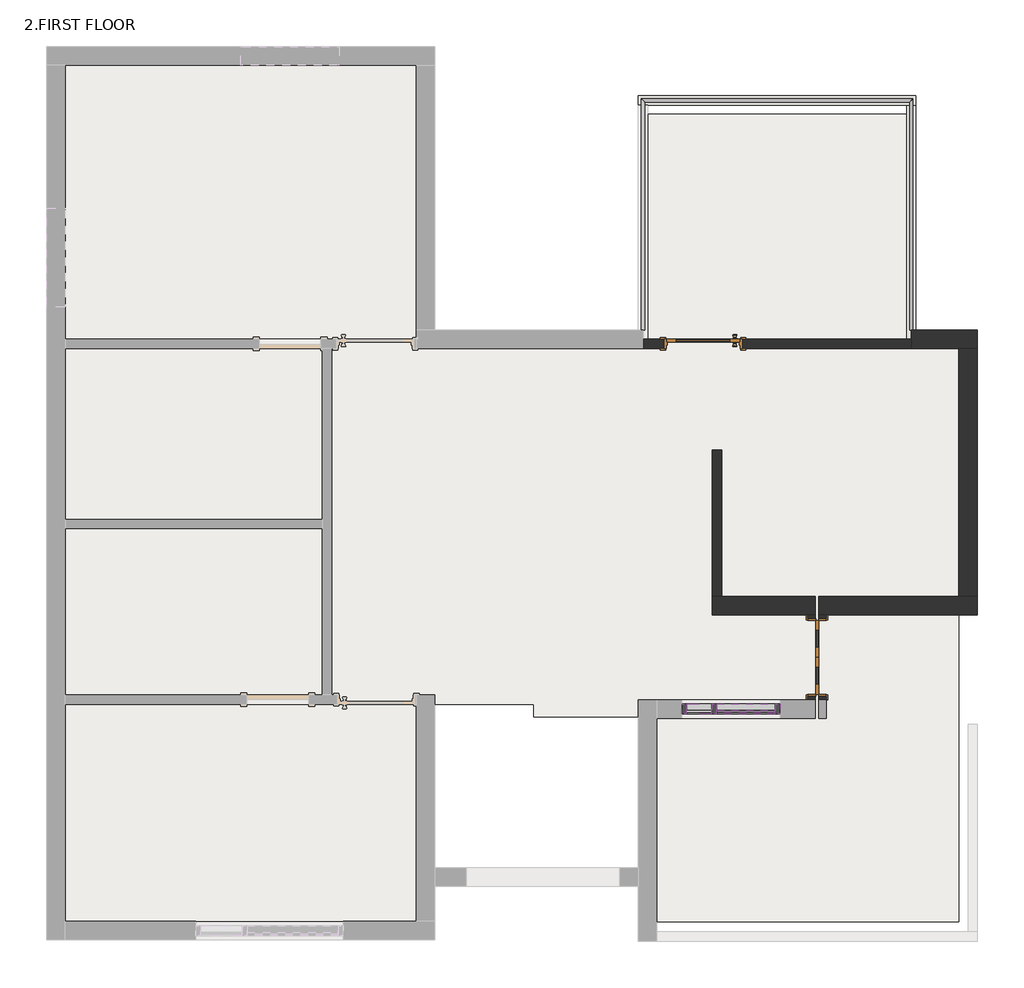
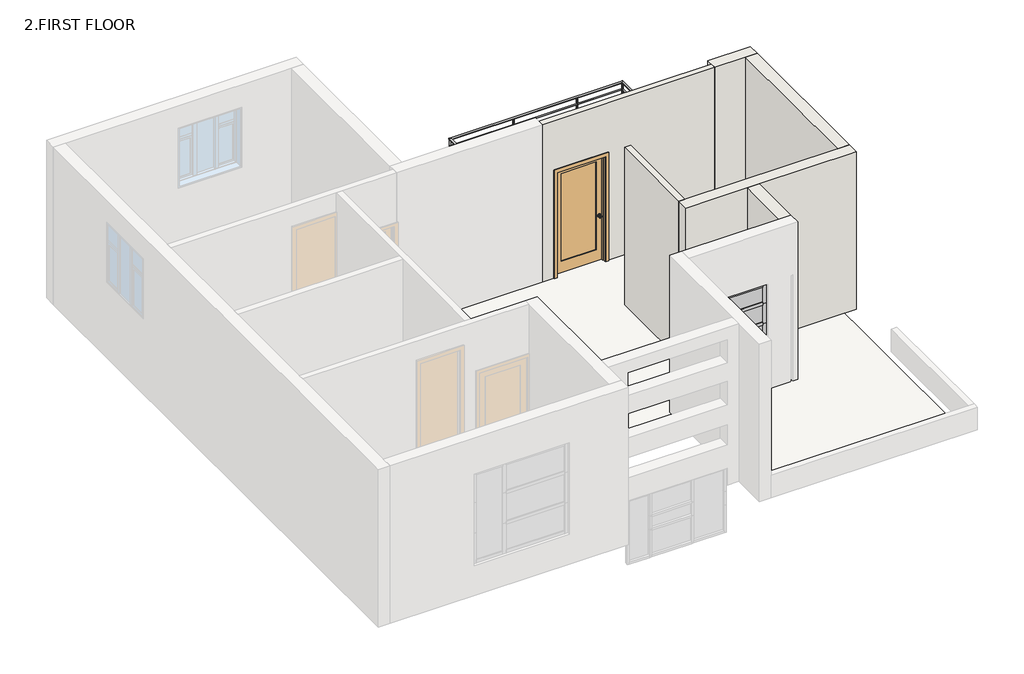
# One storey, part 2 of 2: 15 members, 8 walls, 3 plates, 2 doors, 1 railing, 1 slab.
"""IFC4 building model written with IfcOpenShell, lengths in millimetres."""

from ifc_helpers import new_model, si_unit, point, frame, frame_2d, origin, place, context, project, spatial, polyline, circle_curve, ellipse_curve, trimmed, segment, composite_curve, outline, extrude, faceted_brep, transform, mapped, element, save
from ifc_brep_helpers import plane_surface, cylinder_surface, advanced_brep
from components import door_interior_double_pocket_2_panel_wood_3_x_7_65f9ecc5, door_interior_single_1_panel_wood_4_x7_a3feeac7, member_5ad95953, member_7007ad49, member_90c805a2, member_abeaf8ac, member_7cfea1b5, system_panel_glazed_fef3bb39, system_panel_glazed_ef4f0122

model = new_model("IFC4")

# Units and contexts
model_context = context("Model", 3, world=origin())
ifc_project = project(units=[si_unit("LENGTHUNIT", "METRE", prefix="MILLI")], contexts=[model_context])

# Site, building, storey
site = spatial("IfcSite", under=ifc_project)
building = spatial("IfcBuilding", under=site)
storey = spatial("IfcBuildingStorey", under=building, Name="2.FIRST FLOOR", Elevation=3810.0)

# Doors
placement = place(None, origin())
door_interior_double_pocket_2_panel_wood_3_x_7_shape = door_interior_double_pocket_2_panel_wood_3_x_7_65f9ecc5(model_context)
element("IfcDoor", 1, ObjectType="Door-Interior-Double-Pocket-2_Panel-Wood : 3' x 7'", at=placement, inside=storey, context=model_context, shape_type="MappedRepresentation", body=[
    mapped(door_interior_double_pocket_2_panel_wood_3_x_7_shape, transform((1959.9250448, 2774.2910289, 3810.0), x_axis=(0.0, -1.0, 0.0), y_axis=(1.0, 0.0, 0.0), z_axis=(0.0, 0.0, 1.0))),
])
door_interior_single_1_panel_wood_4_x7_shape = door_interior_single_1_panel_wood_4_x7_a3feeac7(model_context)
element("IfcDoor", 2, ObjectType="Door-Interior-Single-1_Panel-Wood : 4'X7'", at=placement, inside=storey, context=model_context, shape_type="MappedRepresentation", body=[
    mapped(door_interior_single_1_panel_wood_4_x7_shape, transform((550.2250448, 6654.1410289, 3810.0), x_axis=(-1.0, 0.0, 0.0), y_axis=(0.0, -1.0, 0.0), z_axis=(0.0, 0.0, 1.0))),
])

# Members
member_shape = member_5ad95953(model_context)
element("IfcMember", 3, ObjectType="Rectangular Mullion : 2.5\" x 5\" rectangular", at=placement, inside=storey, context=model_context, shape_type="MappedRepresentation", body=[
    mapped(member_shape, transform((347.0250448, 2136.1160289, 5943.6), x_axis=(0.0, 0.0, 1.0), y_axis=(0.0, 1.0, 0.0), z_axis=(-1.0, 0.0, 0.0))),
])
member_2_shape = member_7007ad49(model_context)
element("IfcMember", 4, ObjectType="Rectangular Mullion : 2.5\" x 5\" rectangular", at=placement, inside=storey, context=model_context, shape_type="MappedRepresentation", body=[
    mapped(member_2_shape, transform((1439.2250448, 2136.1160289, 4724.4), x_axis=(0.0, 0.0, -1.0), y_axis=(0.0, 1.0, 0.0), z_axis=(1.0, 0.0, 0.0))),
])
member_3_shape = member_90c805a2(model_context)
element("IfcMember", 5, ObjectType="Rectangular Mullion : 2.5\" x 5\" rectangular", at=placement, inside=storey, context=model_context, shape_type="MappedRepresentation", body=[
    mapped(member_3_shape, transform((689.9250448, 2136.1160289, 4724.4), x_axis=(-1.0, 0.0, 0.0), y_axis=(0.0, 1.0, 0.0), z_axis=(0.0, 0.0, -1.0))),
])
member_4_shape = member_abeaf8ac(model_context)
element("IfcMember", 6, ObjectType="Rectangular Mullion : 2.5\" x 5\" rectangular", at=placement, inside=storey, context=model_context, shape_type="MappedRepresentation", body=[
    mapped(member_4_shape, transform((721.6750448, 2136.1160289, 5537.2), x_axis=(0.0, 0.0, 1.0), y_axis=(0.0, 1.0, 0.0), z_axis=(-1.0, 0.0, 0.0))),
])
element("IfcMember", 7, ObjectType="Rectangular Mullion : 2.5\" x 5\" rectangular", at=placement, inside=storey, context=model_context, shape_type="MappedRepresentation", body=[
    mapped(member_4_shape, transform((721.6750448, 2136.1160289, 5130.8), x_axis=(0.0, 0.0, 1.0), y_axis=(0.0, 1.0, 0.0), z_axis=(-1.0, 0.0, 0.0))),
])
element("IfcMember", 8, ObjectType="Rectangular Mullion : 2.5\" x 5\" rectangular", at=placement, inside=storey, context=model_context, shape_type="MappedRepresentation", body=[
    mapped(member_shape, transform((658.1750448, 2136.1160289, 4724.4), x_axis=(0.0, 0.0, -1.0), y_axis=(0.0, 1.0, 0.0), z_axis=(1.0, 0.0, 0.0))),
])
element("IfcMember", 9, ObjectType="Rectangular Mullion : 2.5\" x 5\" rectangular", at=placement, inside=storey, context=model_context, shape_type="MappedRepresentation", body=[
    mapped(member_2_shape, transform((721.6750448, 2136.1160289, 5943.6), x_axis=(0.0, 0.0, 1.0), y_axis=(0.0, 1.0, 0.0), z_axis=(-1.0, 0.0, 0.0))),
])
element("IfcMember", 10, ObjectType="Rectangular Mullion : 2.5\" x 5\" rectangular", at=placement, inside=storey, context=model_context, shape_type="MappedRepresentation", body=[
    mapped(member_3_shape, transform((689.9250448, 2136.1160289, 5537.2), x_axis=(-1.0, 0.0, 0.0), y_axis=(0.0, 1.0, 0.0), z_axis=(0.0, 0.0, -1.0))),
])
element("IfcMember", 11, ObjectType="Rectangular Mullion : 2.5\" x 5\" rectangular", at=placement, inside=storey, context=model_context, shape_type="MappedRepresentation", body=[
    mapped(member_3_shape, transform((689.9250448, 2136.1160289, 5130.8), x_axis=(-1.0, 0.0, 0.0), y_axis=(0.0, 1.0, 0.0), z_axis=(0.0, 0.0, -1.0))),
])
member_5_shape = member_7cfea1b5(model_context)
element("IfcMember", 12, ObjectType="Rectangular Mullion : 2.5\" x 5\" rectangular", at=placement, inside=storey, context=model_context, shape_type="MappedRepresentation", body=[
    mapped(member_5_shape, transform((1502.7250448, 2136.1160289, 5943.6), x_axis=(1.0, 0.0, 0.0), y_axis=(0.0, 1.0, 0.0), z_axis=(0.0, 0.0, 1.0))),
])
element("IfcMember", 13, ObjectType="Rectangular Mullion : 2.5\" x 5\" rectangular", at=placement, inside=storey, context=model_context, shape_type="MappedRepresentation", body=[
    mapped(member_5_shape, transform((283.5250448, 2136.1160289, 4724.4), x_axis=(-1.0, 0.0, 0.0), y_axis=(0.0, 1.0, 0.0), z_axis=(0.0, 0.0, -1.0))),
])
element("IfcMember", 14, ObjectType="Rectangular Mullion : 2.5\" x 5\" rectangular", at=placement, inside=storey, context=model_context, shape_type="MappedRepresentation", body=[
    mapped(member_5_shape, transform((283.5250448, 2136.1160289, 5537.2), x_axis=(-1.0, 0.0, 0.0), y_axis=(0.0, 1.0, 0.0), z_axis=(0.0, 0.0, -1.0))),
])
element("IfcMember", 15, ObjectType="Rectangular Mullion : 2.5\" x 5\" rectangular", at=placement, inside=storey, context=model_context, shape_type="MappedRepresentation", body=[
    mapped(member_5_shape, transform((283.5250448, 2136.1160289, 5130.8), x_axis=(-1.0, 0.0, 0.0), y_axis=(0.0, 1.0, 0.0), z_axis=(0.0, 0.0, -1.0))),
])
element("IfcMember", 16, ObjectType="Rectangular Mullion : 2.5\" x 5\" rectangular", at=placement, inside=storey, context=model_context, shape_type="MappedRepresentation", body=[
    mapped(member_5_shape, transform((1502.7250448, 2136.1160289, 5537.2), x_axis=(1.0, 0.0, 0.0), y_axis=(0.0, 1.0, 0.0), z_axis=(0.0, 0.0, 1.0))),
])
element("IfcMember", 17, ObjectType="Rectangular Mullion : 2.5\" x 5\" rectangular", at=placement, inside=storey, context=model_context, shape_type="MappedRepresentation", body=[
    mapped(member_5_shape, transform((1502.7250448, 2136.1160289, 5130.8), x_axis=(1.0, 0.0, 0.0), y_axis=(0.0, 1.0, 0.0), z_axis=(0.0, 0.0, 1.0))),
])

# Plates
system_panel_glazed_shape = system_panel_glazed_fef3bb39(model_context)
element("IfcPlate", 18, ObjectType="System Panel : Glazed", at=placement, inside=storey, context=model_context, shape_type="MappedRepresentation", body=[
    mapped(system_panel_glazed_shape, transform((1080.4500448, 2136.1160289, 4787.9), x_axis=(-1.0, 0.0, 0.0), y_axis=(0.0, -1.0, 0.0), z_axis=(0.0, 0.0, 1.0))),
])
element("IfcPlate", 19, ObjectType="System Panel : Glazed", at=placement, inside=storey, context=model_context, shape_type="MappedRepresentation", body=[
    mapped(system_panel_glazed_shape, transform((1080.4500448, 2136.1160289, 5568.95), x_axis=(-1.0, 0.0, 0.0), y_axis=(0.0, -1.0, 0.0), z_axis=(0.0, 0.0, 1.0))),
])
system_panel_glazed_2_shape = system_panel_glazed_ef4f0122(model_context)
element("IfcPlate", 20, ObjectType="System Panel : Glazed", at=placement, inside=storey, context=model_context, shape_type="MappedRepresentation", body=[
    mapped(system_panel_glazed_2_shape, transform((1080.4500448, 2136.1160289, 5162.55), x_axis=(-1.0, 0.0, 0.0), y_axis=(0.0, -1.0, 0.0), z_axis=(0.0, 0.0, 1.0))),
])

# Railing
element("IfcRailing", 21, ObjectType="Handrail - Pipe", at=placement, inside=storey, context=model_context, shape_type="SolidModel", body=[
    advanced_brep(
    [(-173.6749552, 6822.4160289, 4857.75), (-211.7749552, 6822.4160289, 4857.75), (3102.9250448, 6822.4160289, 4857.75), (3141.0250448, 6822.4160289, 4857.75), (-173.6749552, 9641.8160289, 4857.75), (-211.7749552, 9679.9160289, 4857.75), (3102.9250448, 9641.8160289, 4857.75), (3141.0250448, 9679.9160289, 4857.75)],
    [
        (0, 1, circle_curve(frame((-192.7249552, 6822.4160289, 4857.75), z_axis=(0.0, -1.0, 0.0), x_axis=(-1.0, 0.0, 0.0)), 19.05)),
        (1, 0, circle_curve(frame((-192.7249552, 6822.4160289, 4857.75), z_axis=(0.0, -1.0, 0.0), x_axis=(-1.0, 0.0, 0.0)), 19.05)),
        (2, 3, circle_curve(frame((3121.9750448, 6822.4160289, 4857.75), z_axis=(0.0, -1.0, 0.0), x_axis=(1.0, 0.0, 0.0)), 19.05)),
        (3, 2, circle_curve(frame((3121.9750448, 6822.4160289, 4857.75), z_axis=(0.0, -1.0, 0.0), x_axis=(1.0, 0.0, 0.0)), 19.05)),
        (0, 4),
        (4, 5, ellipse_curve(frame((-192.7249552, 9660.8660289, 4857.75), z_axis=(-0.7071067811865492, -0.7071067811865458, 0.0), x_axis=(0.7071067811865457, -0.7071067811865492, 0.0)), 26.9407684, 19.05)),
        (5, 1),
        (5, 4, ellipse_curve(frame((-192.7249552, 9660.8660289, 4857.75), z_axis=(-0.7071067811865492, -0.7071067811865458, 0.0), x_axis=(0.7071067811865457, -0.7071067811865492, 0.0)), 26.9407684, 19.05)),
        (4, 6),
        (6, 7, ellipse_curve(frame((3121.9750448, 9660.8660289, 4857.75), z_axis=(-0.7071067811865457, 0.7071067811865492, 0.0), x_axis=(-0.7071067811865493, -0.7071067811865457, 0.0)), 26.9407684, 19.05)),
        (7, 5),
        (7, 6, ellipse_curve(frame((3121.9750448, 9660.8660289, 4857.75), z_axis=(-0.7071067811865457, 0.7071067811865492, 0.0), x_axis=(-0.7071067811865493, -0.7071067811865457, 0.0)), 26.9407684, 19.05)),
        (6, 2),
        (3, 7),
    ],
    [
        plane_surface(frame((-192.7249552, 6822.4160289, 4876.8), z_axis=(0.0, -1.0, 0.0), x_axis=(0.0, 0.0, 1.0))),
        plane_surface(frame((3121.9750448, 6822.4160289, 4876.8), z_axis=(0.0, -1.0, 0.0), x_axis=(0.0, 0.0, -1.0))),
        cylinder_surface(frame((-192.7249552, 6822.4160289, 4857.75), z_axis=(0.0, -1.0, 0.0), x_axis=(-1.0, 0.0, 0.0)), 19.05),
        cylinder_surface(frame((-192.7249552, 9660.8660289, 4857.75), z_axis=(-1.0, 0.0, 0.0), x_axis=(0.0, 1.0, 0.0)), 19.05),
        cylinder_surface(frame((3121.9750448, 9660.8660289, 4857.75), z_axis=(0.0, 1.0, 0.0), x_axis=(1.0, 0.0, 0.0)), 19.05),
    ],
    [
        (0, [[1, 2]]),
        (1, [[3, 4]]),
        (2, [[-1, 5, 6, 7]]),
        (2, [[-2, -7, 8, -5]]),
        (3, [[-6, 9, 10, 11]]),
        (3, [[-8, -11, 12, -9]]),
        (4, [[-10, 13, -4, 14]]),
        (4, [[-12, -14, -3, -13]]),
    ],
),
    advanced_brep(
    [(-205.4249552, 6822.4160289, 4711.7), (-180.0249552, 6822.4160289, 4711.7), (3134.6750448, 6822.4160289, 4711.7), (3109.2750448, 6822.4160289, 4711.7), (-205.4249552, 9673.5660289, 4711.7), (-180.0249552, 9648.1660289, 4711.7), (3134.6750448, 9673.5660289, 4711.7), (3109.2750448, 9648.1660289, 4711.7)],
    [
        (0, 1, circle_curve(frame((-192.7249552, 6822.4160289, 4711.7), z_axis=(0.0, -1.0, 0.0), x_axis=(1.0, 0.0, 0.0)), 12.7)),
        (1, 0, circle_curve(frame((-192.7249552, 6822.4160289, 4711.7), z_axis=(0.0, -1.0, 0.0), x_axis=(1.0, 0.0, 0.0)), 12.7)),
        (2, 3, circle_curve(frame((3121.9750448, 6822.4160289, 4711.7), z_axis=(0.0, -1.0, 0.0), x_axis=(-1.0, 0.0, 0.0)), 12.7)),
        (3, 2, circle_curve(frame((3121.9750448, 6822.4160289, 4711.7), z_axis=(0.0, -1.0, 0.0), x_axis=(-1.0, 0.0, 0.0)), 12.7)),
        (0, 4),
        (4, 5, ellipse_curve(frame((-192.7249552, 9660.8660289, 4711.7), z_axis=(-0.7071067811865492, -0.7071067811865458, 0.0), x_axis=(0.7071067811865457, -0.7071067811865492, 0.0)), 17.9605122, 12.7)),
        (5, 1),
        (5, 4, ellipse_curve(frame((-192.7249552, 9660.8660289, 4711.7), z_axis=(-0.7071067811865492, -0.7071067811865458, 0.0), x_axis=(0.7071067811865457, -0.7071067811865492, 0.0)), 17.9605122, 12.7)),
        (4, 6),
        (6, 7, ellipse_curve(frame((3121.9750448, 9660.8660289, 4711.7), z_axis=(-0.7071067811865457, 0.7071067811865492, 0.0), x_axis=(-0.7071067811865493, -0.7071067811865457, 0.0)), 17.9605122, 12.7)),
        (7, 5),
        (7, 6, ellipse_curve(frame((3121.9750448, 9660.8660289, 4711.7), z_axis=(-0.7071067811865457, 0.7071067811865492, 0.0), x_axis=(-0.7071067811865493, -0.7071067811865457, 0.0)), 17.9605122, 12.7)),
        (6, 2),
        (3, 7),
    ],
    [
        plane_surface(frame((-192.7249552, 6822.4160289, 4724.4), z_axis=(0.0, -1.0, 0.0), x_axis=(0.0, 0.0, 1.0))),
        plane_surface(frame((3121.9750448, 6822.4160289, 4724.4), z_axis=(0.0, -1.0, 0.0), x_axis=(0.0, 0.0, -1.0))),
        cylinder_surface(frame((-192.7249552, 6822.4160289, 4711.7), z_axis=(0.0, -1.0, 0.0), x_axis=(1.0, 0.0, 0.0)), 12.7),
        cylinder_surface(frame((-192.7249552, 9660.8660289, 4711.7), z_axis=(-1.0, 0.0, 0.0), x_axis=(0.0, -1.0, 0.0)), 12.7),
        cylinder_surface(frame((3121.9750448, 9660.8660289, 4711.7), z_axis=(0.0, 1.0, 0.0), x_axis=(-1.0, 0.0, 0.0)), 12.7),
    ],
    [
        (0, [[1, 2]]),
        (1, [[3, 4]]),
        (2, [[-1, 5, 6, 7]]),
        (2, [[-2, -7, 8, -5]]),
        (3, [[-6, 9, 10, 11]]),
        (3, [[-8, -11, 12, -9]]),
        (4, [[-10, 13, -4, 14]]),
        (4, [[-12, -14, -3, -13]]),
    ],
),
    advanced_brep(
    [(-205.4249552, 6822.4160289, 4559.3), (-180.0249552, 6822.4160289, 4559.3), (3134.6750448, 6822.4160289, 4559.3), (3109.2750448, 6822.4160289, 4559.3), (-205.4249552, 9673.5660289, 4559.3), (-180.0249552, 9648.1660289, 4559.3), (3134.6750448, 9673.5660289, 4559.3), (3109.2750448, 9648.1660289, 4559.3)],
    [
        (0, 1, circle_curve(frame((-192.7249552, 6822.4160289, 4559.3), z_axis=(0.0, -1.0, 0.0), x_axis=(1.0, 0.0, 0.0)), 12.7)),
        (1, 0, circle_curve(frame((-192.7249552, 6822.4160289, 4559.3), z_axis=(0.0, -1.0, 0.0), x_axis=(1.0, 0.0, 0.0)), 12.7)),
        (2, 3, circle_curve(frame((3121.9750448, 6822.4160289, 4559.3), z_axis=(0.0, -1.0, 0.0), x_axis=(-1.0, 0.0, 0.0)), 12.7)),
        (3, 2, circle_curve(frame((3121.9750448, 6822.4160289, 4559.3), z_axis=(0.0, -1.0, 0.0), x_axis=(-1.0, 0.0, 0.0)), 12.7)),
        (0, 4),
        (4, 5, ellipse_curve(frame((-192.7249552, 9660.8660289, 4559.3), z_axis=(-0.7071067811865492, -0.7071067811865458, 0.0), x_axis=(0.7071067811865457, -0.7071067811865492, 0.0)), 17.9605122, 12.7)),
        (5, 1),
        (5, 4, ellipse_curve(frame((-192.7249552, 9660.8660289, 4559.3), z_axis=(-0.7071067811865492, -0.7071067811865458, 0.0), x_axis=(0.7071067811865457, -0.7071067811865492, 0.0)), 17.9605122, 12.7)),
        (4, 6),
        (6, 7, ellipse_curve(frame((3121.9750448, 9660.8660289, 4559.3), z_axis=(-0.7071067811865457, 0.7071067811865492, 0.0), x_axis=(-0.7071067811865493, -0.7071067811865457, 0.0)), 17.9605122, 12.7)),
        (7, 5),
        (7, 6, ellipse_curve(frame((3121.9750448, 9660.8660289, 4559.3), z_axis=(-0.7071067811865457, 0.7071067811865492, 0.0), x_axis=(-0.7071067811865493, -0.7071067811865457, 0.0)), 17.9605122, 12.7)),
        (6, 2),
        (3, 7),
    ],
    [
        plane_surface(frame((-192.7249552, 6822.4160289, 4572.0), z_axis=(0.0, -1.0, 0.0), x_axis=(0.0, 0.0, 1.0))),
        plane_surface(frame((3121.9750448, 6822.4160289, 4572.0), z_axis=(0.0, -1.0, 0.0), x_axis=(0.0, 0.0, -1.0))),
        cylinder_surface(frame((-192.7249552, 6822.4160289, 4559.3), z_axis=(0.0, -1.0, 0.0), x_axis=(1.0, 0.0, 0.0)), 12.7),
        cylinder_surface(frame((-192.7249552, 9660.8660289, 4559.3), z_axis=(-1.0, 0.0, 0.0), x_axis=(0.0, -1.0, 0.0)), 12.7),
        cylinder_surface(frame((3121.9750448, 9660.8660289, 4559.3), z_axis=(0.0, 1.0, 0.0), x_axis=(-1.0, 0.0, 0.0)), 12.7),
    ],
    [
        (0, [[1, 2]]),
        (1, [[3, 4]]),
        (2, [[-1, 5, 6, 7]]),
        (2, [[-2, -7, 8, -5]]),
        (3, [[-6, 9, 10, 11]]),
        (3, [[-8, -11, 12, -9]]),
        (4, [[-10, 13, -4, 14]]),
        (4, [[-12, -14, -3, -13]]),
    ],
),
    advanced_brep(
    [(-205.4249552, 6822.4160289, 4406.9), (-180.0249552, 6822.4160289, 4406.9), (-205.4249552, 9673.5660289, 4406.9), (-180.0249552, 9648.1660289, 4406.9), (3134.6750448, 9673.5660289, 4406.9), (3109.2750448, 9648.1660289, 4406.9), (3134.6750448, 6822.4160289, 4406.9), (3109.2750448, 6822.4160289, 4406.9)],
    [
        (0, 1, circle_curve(frame((-192.7249552, 6822.4160289, 4406.9), z_axis=(0.0, -1.0, 0.0), x_axis=(1.0, 0.0, 0.0)), 12.7)),
        (1, 0, circle_curve(frame((-192.7249552, 6822.4160289, 4406.9), z_axis=(0.0, -1.0, 0.0), x_axis=(1.0, 0.0, 0.0)), 12.7)),
        (0, 2),
        (2, 3, ellipse_curve(frame((-192.7249552, 9660.8660289, 4406.9), z_axis=(-0.7071067811865492, -0.7071067811865458, 0.0), x_axis=(0.7071067811865457, -0.7071067811865492, 0.0)), 17.9605122, 12.7)),
        (3, 1),
        (3, 2, ellipse_curve(frame((-192.7249552, 9660.8660289, 4406.9), z_axis=(-0.7071067811865492, -0.7071067811865458, 0.0), x_axis=(0.7071067811865457, -0.7071067811865492, 0.0)), 17.9605122, 12.7)),
        (2, 4),
        (4, 5, ellipse_curve(frame((3121.9750448, 9660.8660289, 4406.9), z_axis=(-0.7071067811865457, 0.7071067811865492, 0.0), x_axis=(-0.7071067811865493, -0.7071067811865457, 0.0)), 17.9605122, 12.7)),
        (5, 3),
        (5, 4, ellipse_curve(frame((3121.9750448, 9660.8660289, 4406.9), z_axis=(-0.7071067811865457, 0.7071067811865492, 0.0), x_axis=(-0.7071067811865493, -0.7071067811865457, 0.0)), 17.9605122, 12.7)),
        (6, 7, circle_curve(frame((3121.9750448, 6822.4160289, 4406.9), z_axis=(0.0, -1.0, 0.0), x_axis=(-1.0, 0.0, 0.0)), 12.7)),
        (7, 6, circle_curve(frame((3121.9750448, 6822.4160289, 4406.9), z_axis=(0.0, -1.0, 0.0), x_axis=(-1.0, 0.0, 0.0)), 12.7)),
        (4, 6),
        (7, 5),
    ],
    [
        plane_surface(frame((-192.7249552, 6822.4160289, 4419.6), z_axis=(0.0, -1.0, 0.0), x_axis=(0.0, 0.0, 1.0))),
        cylinder_surface(frame((-192.7249552, 6822.4160289, 4406.9), z_axis=(0.0, -1.0, 0.0), x_axis=(1.0, 0.0, 0.0)), 12.7),
        cylinder_surface(frame((-192.7249552, 9660.8660289, 4406.9), z_axis=(-1.0, 0.0, 0.0), x_axis=(0.0, -1.0, 0.0)), 12.7),
        plane_surface(frame((3121.9750448, 6822.4160289, 4419.6), z_axis=(0.0, -1.0, 0.0), x_axis=(0.0, 0.0, -1.0))),
        cylinder_surface(frame((3121.9750448, 9660.8660289, 4406.9), z_axis=(0.0, 1.0, 0.0), x_axis=(-1.0, 0.0, 0.0)), 12.7),
    ],
    [
        (0, [[1, 2]]),
        (1, [[-1, 3, 4, 5]]),
        (1, [[-2, -5, 6, -3]]),
        (2, [[-4, 7, 8, 9]]),
        (2, [[-6, -9, 10, -7]]),
        (3, [[11, 12]]),
        (4, [[-8, 13, -12, 14]]),
        (4, [[-10, -14, -11, -13]]),
    ],
),
    advanced_brep(
    [(-205.4249552, 6822.4160289, 4254.5), (-180.0249552, 6822.4160289, 4254.5), (-205.4249552, 9673.5660289, 4254.5), (-180.0249552, 9648.1660289, 4254.5), (3134.6750448, 9673.5660289, 4254.5), (3109.2750448, 9648.1660289, 4254.5), (3134.6750448, 6822.4160289, 4254.5), (3109.2750448, 6822.4160289, 4254.5)],
    [
        (0, 1, circle_curve(frame((-192.7249552, 6822.4160289, 4254.5), z_axis=(0.0, -1.0, 0.0), x_axis=(1.0, 0.0, 0.0)), 12.7)),
        (1, 0, circle_curve(frame((-192.7249552, 6822.4160289, 4254.5), z_axis=(0.0, -1.0, 0.0), x_axis=(1.0, 0.0, 0.0)), 12.7)),
        (0, 2),
        (2, 3, ellipse_curve(frame((-192.7249552, 9660.8660289, 4254.5), z_axis=(-0.7071067811865492, -0.7071067811865458, 0.0), x_axis=(0.7071067811865457, -0.7071067811865492, 0.0)), 17.9605122, 12.7)),
        (3, 1),
        (3, 2, ellipse_curve(frame((-192.7249552, 9660.8660289, 4254.5), z_axis=(-0.7071067811865492, -0.7071067811865458, 0.0), x_axis=(0.7071067811865457, -0.7071067811865492, 0.0)), 17.9605122, 12.7)),
        (2, 4),
        (4, 5, ellipse_curve(frame((3121.9750448, 9660.8660289, 4254.5), z_axis=(-0.7071067811865457, 0.7071067811865492, 0.0), x_axis=(-0.7071067811865493, -0.7071067811865457, 0.0)), 17.9605122, 12.7)),
        (5, 3),
        (5, 4, ellipse_curve(frame((3121.9750448, 9660.8660289, 4254.5), z_axis=(-0.7071067811865457, 0.7071067811865492, 0.0), x_axis=(-0.7071067811865493, -0.7071067811865457, 0.0)), 17.9605122, 12.7)),
        (6, 7, circle_curve(frame((3121.9750448, 6822.4160289, 4254.5), z_axis=(0.0, -1.0, 0.0), x_axis=(-1.0, 0.0, 0.0)), 12.7)),
        (7, 6, circle_curve(frame((3121.9750448, 6822.4160289, 4254.5), z_axis=(0.0, -1.0, 0.0), x_axis=(-1.0, 0.0, 0.0)), 12.7)),
        (4, 6),
        (7, 5),
    ],
    [
        plane_surface(frame((-192.7249552, 6822.4160289, 4267.2), z_axis=(0.0, -1.0, 0.0), x_axis=(0.0, 0.0, 1.0))),
        cylinder_surface(frame((-192.7249552, 6822.4160289, 4254.5), z_axis=(0.0, -1.0, 0.0), x_axis=(1.0, 0.0, 0.0)), 12.7),
        cylinder_surface(frame((-192.7249552, 9660.8660289, 4254.5), z_axis=(-1.0, 0.0, 0.0), x_axis=(0.0, -1.0, 0.0)), 12.7),
        plane_surface(frame((3121.9750448, 6822.4160289, 4267.2), z_axis=(0.0, -1.0, 0.0), x_axis=(0.0, 0.0, -1.0))),
        cylinder_surface(frame((3121.9750448, 9660.8660289, 4254.5), z_axis=(0.0, 1.0, 0.0), x_axis=(-1.0, 0.0, 0.0)), 12.7),
    ],
    [
        (0, [[1, 2]]),
        (1, [[-1, 3, 4, 5]]),
        (1, [[-2, -5, 6, -3]]),
        (2, [[-4, 7, 8, 9]]),
        (2, [[-6, -9, 10, -7]]),
        (3, [[11, 12]]),
        (4, [[-8, 13, -12, 14]]),
        (4, [[-10, -14, -11, -13]]),
    ],
),
    advanced_brep(
    [(-205.4249552, 6822.4160289, 4102.1), (-180.0249552, 6822.4160289, 4102.1), (-205.4249552, 9673.5660289, 4102.1), (-180.0249552, 9648.1660289, 4102.1), (3134.6750448, 9673.5660289, 4102.1), (3109.2750448, 9648.1660289, 4102.1), (3134.6750448, 6822.4160289, 4102.1), (3109.2750448, 6822.4160289, 4102.1)],
    [
        (0, 1, circle_curve(frame((-192.7249552, 6822.4160289, 4102.1), z_axis=(0.0, -1.0, 0.0), x_axis=(1.0, 0.0, 0.0)), 12.7)),
        (1, 0, circle_curve(frame((-192.7249552, 6822.4160289, 4102.1), z_axis=(0.0, -1.0, 0.0), x_axis=(1.0, 0.0, 0.0)), 12.7)),
        (0, 2),
        (2, 3, ellipse_curve(frame((-192.7249552, 9660.8660289, 4102.1), z_axis=(-0.7071067811865492, -0.7071067811865458, 0.0), x_axis=(0.7071067811865457, -0.7071067811865492, 0.0)), 17.9605122, 12.7)),
        (3, 1),
        (3, 2, ellipse_curve(frame((-192.7249552, 9660.8660289, 4102.1), z_axis=(-0.7071067811865492, -0.7071067811865458, 0.0), x_axis=(0.7071067811865457, -0.7071067811865492, 0.0)), 17.9605122, 12.7)),
        (2, 4),
        (4, 5, ellipse_curve(frame((3121.9750448, 9660.8660289, 4102.1), z_axis=(-0.7071067811865457, 0.7071067811865492, 0.0), x_axis=(-0.7071067811865493, -0.7071067811865457, 0.0)), 17.9605122, 12.7)),
        (5, 3),
        (5, 4, ellipse_curve(frame((3121.9750448, 9660.8660289, 4102.1), z_axis=(-0.7071067811865457, 0.7071067811865492, 0.0), x_axis=(-0.7071067811865493, -0.7071067811865457, 0.0)), 17.9605122, 12.7)),
        (6, 7, circle_curve(frame((3121.9750448, 6822.4160289, 4102.1), z_axis=(0.0, -1.0, 0.0), x_axis=(-1.0, 0.0, 0.0)), 12.7)),
        (7, 6, circle_curve(frame((3121.9750448, 6822.4160289, 4102.1), z_axis=(0.0, -1.0, 0.0), x_axis=(-1.0, 0.0, 0.0)), 12.7)),
        (4, 6),
        (7, 5),
    ],
    [
        plane_surface(frame((-192.7249552, 6822.4160289, 4114.8), z_axis=(0.0, -1.0, 0.0), x_axis=(0.0, 0.0, 1.0))),
        cylinder_surface(frame((-192.7249552, 6822.4160289, 4102.1), z_axis=(0.0, -1.0, 0.0), x_axis=(1.0, 0.0, 0.0)), 12.7),
        cylinder_surface(frame((-192.7249552, 9660.8660289, 4102.1), z_axis=(-1.0, 0.0, 0.0), x_axis=(0.0, -1.0, 0.0)), 12.7),
        plane_surface(frame((3121.9750448, 6822.4160289, 4114.8), z_axis=(0.0, -1.0, 0.0), x_axis=(0.0, 0.0, -1.0))),
        cylinder_surface(frame((3121.9750448, 9660.8660289, 4102.1), z_axis=(0.0, 1.0, 0.0), x_axis=(-1.0, 0.0, 0.0)), 12.7),
    ],
    [
        (0, [[1, 2]]),
        (1, [[-1, 3, 4, 5]]),
        (1, [[-2, -5, 6, -3]]),
        (2, [[-4, 7, 8, 9]]),
        (2, [[-6, -9, 10, -7]]),
        (3, [[11, 12]]),
        (4, [[-8, 13, -12, 14]]),
        (4, [[-10, -14, -11, -13]]),
    ],
),
    extrude(outline(composite_curve([segment(trimmed(circle_curve(frame_2d((3121.9750448, 7222.4660289)), 12.7), [point((3134.6750448, 7222.4660289))], [point((3109.2750448, 7222.4660289))], False, "CARTESIAN"), True, "CONTINUOUS"), segment(trimmed(circle_curve(frame_2d((3121.9750448, 7222.4660289)), 12.7), [point((3109.2750448, 7222.4660289))], [point((3134.6750448, 7222.4660289))], False, "CARTESIAN"), True, "CONTINUOUS")], self_intersect=False)), frame((0.0, 0.0, 3962.4), z_axis=(0.0, 0.0, 1.0), x_axis=(1.0, 0.0, 0.0)), (0.0, 0.0, 1.0), 876.3),
    extrude(outline(composite_curve([segment(trimmed(circle_curve(frame_2d((3121.9750448, 8441.6660289)), 12.7), [point((3134.6750448, 8441.6660289))], [point((3109.2750448, 8441.6660289))], False, "CARTESIAN"), True, "CONTINUOUS"), segment(trimmed(circle_curve(frame_2d((3121.9750448, 8441.6660289)), 12.7), [point((3109.2750448, 8441.6660289))], [point((3134.6750448, 8441.6660289))], False, "CARTESIAN"), True, "CONTINUOUS")], self_intersect=False)), frame((0.0, 0.0, 3962.4), z_axis=(0.0, 0.0, 1.0), x_axis=(1.0, 0.0, 0.0)), (0.0, 0.0, 1.0), 876.3),
    extrude(outline(composite_curve([segment(trimmed(circle_curve(frame_2d((2245.6750448, 9660.8660289)), 12.7), [point((2245.6750448, 9673.5660289))], [point((2245.6750448, 9648.1660289))], False, "CARTESIAN"), True, "CONTINUOUS"), segment(trimmed(circle_curve(frame_2d((2245.6750448, 9660.8660289)), 12.7), [point((2245.6750448, 9648.1660289))], [point((2245.6750448, 9673.5660289))], False, "CARTESIAN"), True, "CONTINUOUS")], self_intersect=False)), frame((0.0, 0.0, 3962.4), z_axis=(0.0, 0.0, 1.0), x_axis=(1.0, 0.0, 0.0)), (0.0, 0.0, 1.0), 876.3),
    extrude(outline(composite_curve([segment(trimmed(circle_curve(frame_2d((1026.4750448, 9660.8660289)), 12.7), [point((1026.4750448, 9673.5660289))], [point((1026.4750448, 9648.1660289))], False, "CARTESIAN"), True, "CONTINUOUS"), segment(trimmed(circle_curve(frame_2d((1026.4750448, 9660.8660289)), 12.7), [point((1026.4750448, 9648.1660289))], [point((1026.4750448, 9673.5660289))], False, "CARTESIAN"), True, "CONTINUOUS")], self_intersect=False)), frame((0.0, 0.0, 3962.4), z_axis=(0.0, 0.0, 1.0), x_axis=(1.0, 0.0, 0.0)), (0.0, 0.0, 1.0), 876.3),
    extrude(outline(composite_curve([segment(trimmed(circle_curve(frame_2d((-192.7249552, 9260.8160289)), 12.7), [point((-205.4249552, 9260.8160289))], [point((-180.0249552, 9260.8160289))], False, "CARTESIAN"), True, "CONTINUOUS"), segment(trimmed(circle_curve(frame_2d((-192.7249552, 9260.8160289)), 12.7), [point((-180.0249552, 9260.8160289))], [point((-205.4249552, 9260.8160289))], False, "CARTESIAN"), True, "CONTINUOUS")], self_intersect=False)), frame((0.0, 0.0, 3962.4), z_axis=(0.0, 0.0, 1.0), x_axis=(1.0, 0.0, 0.0)), (0.0, 0.0, 1.0), 876.3),
    extrude(outline(composite_curve([segment(trimmed(circle_curve(frame_2d((-192.7249552, 8041.6160289)), 12.7), [point((-205.4249552, 8041.6160289))], [point((-180.0249552, 8041.6160289))], False, "CARTESIAN"), True, "CONTINUOUS"), segment(trimmed(circle_curve(frame_2d((-192.7249552, 8041.6160289)), 12.7), [point((-180.0249552, 8041.6160289))], [point((-205.4249552, 8041.6160289))], False, "CARTESIAN"), True, "CONTINUOUS")], self_intersect=False)), frame((0.0, 0.0, 3962.4), z_axis=(0.0, 0.0, 1.0), x_axis=(1.0, 0.0, 0.0)), (0.0, 0.0, 1.0), 876.3),
    extrude(outline(composite_curve([segment(trimmed(circle_curve(frame_2d((3121.9750448, 9660.8660289)), 12.7), [point((3121.9750448, 9673.5660289))], [point((3121.9750448, 9648.1660289))], False, "CARTESIAN"), True, "CONTINUOUS"), segment(trimmed(circle_curve(frame_2d((3121.9750448, 9660.8660289)), 12.7), [point((3121.9750448, 9648.1660289))], [point((3121.9750448, 9673.5660289))], False, "CARTESIAN"), True, "CONTINUOUS")], self_intersect=False)), frame((0.0, 0.0, 3962.4), z_axis=(0.0, 0.0, 1.0), x_axis=(1.0, 0.0, 0.0)), (0.0, 0.0, 1.0), 876.3),
    extrude(outline(composite_curve([segment(trimmed(circle_curve(frame_2d((-192.7249552, 9660.8660289)), 12.7), [point((-205.4249552, 9660.8660289))], [point((-180.0249552, 9660.8660289))], False, "CARTESIAN"), True, "CONTINUOUS"), segment(trimmed(circle_curve(frame_2d((-192.7249552, 9660.8660289)), 12.7), [point((-180.0249552, 9660.8660289))], [point((-205.4249552, 9660.8660289))], False, "CARTESIAN"), True, "CONTINUOUS")], self_intersect=False)), frame((0.0, 0.0, 3962.4), z_axis=(0.0, 0.0, 1.0), x_axis=(1.0, 0.0, 0.0)), (0.0, 0.0, 1.0), 876.3),
    extrude(outline(composite_curve([segment(trimmed(circle_curve(frame_2d((3121.9750448, 6835.1160289)), 12.7), [point((3134.6750448, 6835.1160289))], [point((3109.2750448, 6835.1160289))], False, "CARTESIAN"), True, "CONTINUOUS"), segment(trimmed(circle_curve(frame_2d((3121.9750448, 6835.1160289)), 12.7), [point((3109.2750448, 6835.1160289))], [point((3134.6750448, 6835.1160289))], False, "CARTESIAN"), True, "CONTINUOUS")], self_intersect=False)), frame((0.0, 0.0, 3962.4), z_axis=(0.0, 0.0, 1.0), x_axis=(1.0, 0.0, 0.0)), (0.0, 0.0, 1.0), 876.3),
    extrude(outline(composite_curve([segment(trimmed(circle_curve(frame_2d((-192.7249552, 6835.1160289)), 12.7), [point((-205.4249552, 6835.1160289))], [point((-180.0249552, 6835.1160289))], False, "CARTESIAN"), True, "CONTINUOUS"), segment(trimmed(circle_curve(frame_2d((-192.7249552, 6835.1160289)), 12.7), [point((-180.0249552, 6835.1160289))], [point((-205.4249552, 6835.1160289))], False, "CARTESIAN"), True, "CONTINUOUS")], self_intersect=False)), frame((0.0, 0.0, 3962.4), z_axis=(0.0, 0.0, 1.0), x_axis=(1.0, 0.0, 0.0)), (0.0, 0.0, 1.0), 876.3),
])

# Slab
element("IfcSlab", 22, ObjectType="6\" FLOOR", at=placement, inside=storey, context=model_context, shape_type="SweptSolid", body=[
    extrude(outline(polyline([(-2993.0749552, 10099.0160289), (-2993.0749552, 6593.8160289), (-135.5749552, 6593.8160289), (-135.5749552, 9489.4160289), (3064.8250448, 9489.4160289), (3064.8250448, 6708.1160289), (3064.8250448, 6593.8160289), (3712.5250448, 6593.8160289), (3712.5250448, -492.7839711), (-21.2749552, -492.7839711), (-21.2749552, -167.9785909), (-21.2749552, 2040.8660289), (-1545.2749552, 2040.8660289), (-1545.2749552, 2193.2660289), (-2993.0749552, 2193.2660289), (-2993.0749552, -35.5839711), (-2993.0749552, -492.7839711), (-7336.4749552, -492.7839711), (-7336.4749552, 10099.0160289), (-2993.0749552, 10099.0160289)])), frame((0.0, 0.0, 3657.6), z_axis=(0.0, 0.0, 1.0), x_axis=(1.0, 0.0, 0.0)), (0.0, 0.0, 1.0), 152.4),
])

# Walls
element("IfcWall", 23, ObjectType="4.5\" wall", at=placement, inside=storey, context=model_context, shape_type="Brep", body=[
    faceted_brep([(-192.7249552, 6708.1160289, 7010.4), (-135.5749552, 6708.1160289, 7010.4), (3121.9750448, 6708.1160289, 7010.4), (3121.9750448, 6708.1160289, 4114.8), (3121.9750448, 6708.1160289, 3810.0), (3064.8250448, 6708.1160289, 3810.0), (1032.8250448, 6708.1160289, 3810.0), (1032.8250448, 6708.1160289, 5969.0), (67.6250448, 6708.1160289, 5969.0), (67.6250448, 6708.1160289, 3810.0), (-135.5749552, 6708.1160289, 3810.0), (-192.7249552, 6708.1160289, 3810.0), (-192.7249552, 6708.1160289, 4114.8), (-192.7249552, 6708.1160289, 6553.2), (3121.9750448, 6593.8160289, 7010.4), (-192.7249552, 6593.8160289, 7010.4), (-192.7249552, 6593.8160289, 3810.0), (67.6250448, 6593.8160289, 3810.0), (67.6250448, 6593.8160289, 5969.0), (1032.8250448, 6593.8160289, 5969.0), (1032.8250448, 6593.8160289, 3810.0), (3121.9750448, 6593.8160289, 3810.0)], [[[0, 1, 2, 3, 4, 5, 6, 7, 8, 9, 10, 11, 12, 13]], [[14, 15, 16, 17, 18, 19, 20, 21]], [[16, 11, 10, 9, 17]], [[4, 21, 20, 6, 5]], [[2, 1, 0, 15, 14]], [[8, 18, 17, 9]], [[18, 8, 7, 19]], [[19, 7, 6, 20]], [[2, 14, 21, 4, 3]], [[11, 16, 15, 0, 13, 12]]]),
])
element("IfcWall", 24, ObjectType="4.5\" wall", at=placement, inside=storey, context=model_context, shape_type="SweptSolid", body=[
    extrude(outline(polyline([(778.8250448, 5336.5160289), (778.8250448, 3526.7660289), (664.5250448, 3526.7660289), (664.5250448, 5336.5160289), (778.8250448, 5336.5160289)])), frame((0.0, 0.0, 3810.0), z_axis=(0.0, 0.0, 1.0), x_axis=(1.0, 0.0, 0.0)), (0.0, 0.0, 1.0), 3200.4),
])
element("IfcWall", 25, ObjectType="4.5\" wall", at=placement, inside=storey, context=model_context, shape_type="Brep", body=[
    faceted_brep([(-249.8749552, 9603.7160289, 3810.0), (-135.5749552, 9603.7160289, 3810.0), (3064.8250448, 9603.7160289, 3810.0), (3179.1250448, 9603.7160289, 3810.0), (3179.1250448, 9603.7160289, 4114.8), (3064.8250448, 9603.7160289, 4114.8), (-135.5749552, 9603.7160289, 4114.8), (-249.8749552, 9603.7160289, 4114.8), (-249.8749552, 9718.0160289, 3810.0), (-249.8749552, 9718.0160289, 4114.8), (3179.1250448, 9718.0160289, 4114.8), (3179.1250448, 9718.0160289, 3810.0)], [[[0, 1, 2, 3, 4, 5, 6, 7]], [[8, 9, 10, 11]], [[3, 2, 1, 0, 8, 11]], [[7, 6, 5, 4, 10, 9]], [[4, 3, 11, 10]], [[0, 7, 9, 8]]]),
])
element("IfcWall", 26, ObjectType="4.5\" wall", at=placement, inside=storey, context=model_context, shape_type="SweptSolid", body=[
    extrude(outline(polyline([(3064.8250448, 6708.1160289), (3064.8250448, 9603.7160289), (3179.1250448, 9603.7160289), (3179.1250448, 6822.4160289), (3121.9750448, 6822.4160289), (3121.9750448, 6708.1160289), (3064.8250448, 6708.1160289)])), frame((0.0, 0.0, 3810.0), z_axis=(0.0, 0.0, 1.0), x_axis=(1.0, 0.0, 0.0)), (0.0, 0.0, 1.0), 304.8),
])
element("IfcWall", 27, ObjectType="9\" wall", at=placement, inside=storey, context=model_context, shape_type="Brep", body=[
    faceted_brep([(664.5250448, 3526.7660289, 7010.4), (778.8250448, 3526.7660289, 7010.4), (3712.5250448, 3526.7660289, 7010.4), (3941.1250448, 3526.7660289, 7010.4), (3941.1250448, 3526.7660289, 3810.0), (3712.5250448, 3526.7660289, 3810.0), (1980.5625448, 3526.7660289, 3810.0), (1980.5625448, 3526.7660289, 5969.0), (1939.2875448, 3526.7660289, 5969.0), (1939.2875448, 3526.7660289, 3810.0), (778.8250448, 3526.7660289, 3810.0), (664.5250448, 3526.7660289, 3810.0), (3941.1250448, 3298.1660289, 7010.4), (2074.2250448, 3298.1660289, 7010.4), (1845.6250448, 3298.1660289, 7010.4), (664.5250448, 3298.1660289, 7010.4), (664.5250448, 3298.1660289, 3810.0), (1845.6250448, 3298.1660289, 3810.0), (1939.2875448, 3298.1660289, 3810.0), (1939.2875448, 3298.1660289, 5969.0), (1980.5625448, 3298.1660289, 5969.0), (1980.5625448, 3298.1660289, 3810.0), (2074.2250448, 3298.1660289, 3810.0), (3941.1250448, 3298.1660289, 3810.0)], [[[0, 1, 2, 3, 4, 5, 6, 7, 8, 9, 10, 11]], [[12, 13, 14, 15, 16, 17, 18, 19, 20, 21, 22, 23]], [[16, 11, 10, 9, 18, 17]], [[6, 5, 4, 23, 22, 21]], [[3, 2, 1, 0, 15, 14, 13, 12]], [[0, 11, 16, 15]], [[19, 8, 7, 20]], [[20, 7, 6, 21]], [[8, 19, 18, 9]], [[4, 3, 12, 23]]]),
])
element("IfcWall", 28, ObjectType="9\" wall", at=placement, inside=storey, context=model_context, shape_type="Brep", body=[
    faceted_brep([(2074.2250448, 3298.1660289, 7010.4), (2074.2250448, 2250.4160289, 7010.4), (2074.2250448, 2250.4160289, 3810.0), (2074.2250448, 2291.6910289, 3810.0), (2074.2250448, 2291.6910289, 5969.0), (2074.2250448, 3256.8910289, 5969.0), (2074.2250448, 3256.8910289, 3810.0), (2074.2250448, 3298.1660289, 3810.0), (1845.6250448, 2250.4160289, 7010.4), (1845.6250448, 3298.1660289, 7010.4), (1845.6250448, 3298.1660289, 3810.0), (1845.6250448, 3256.8910289, 3810.0), (1845.6250448, 3256.8910289, 5969.0), (1845.6250448, 2291.6910289, 5969.0), (1845.6250448, 2291.6910289, 3810.0), (1845.6250448, 2250.4160289, 3810.0), (1980.5625448, 2250.4160289, 3810.0), (1980.5625448, 2291.6910289, 3810.0), (1980.5625448, 3256.8910289, 3810.0), (1980.5625448, 3298.1660289, 3810.0), (1939.2875448, 3298.1660289, 3810.0), (1939.2875448, 3256.8910289, 3810.0), (1939.2875448, 2291.6910289, 3810.0), (1939.2875448, 2250.4160289, 3810.0), (1939.2875448, 2250.4160289, 5969.0), (1980.5625448, 2250.4160289, 5969.0), (1980.5625448, 3298.1660289, 5969.0), (1939.2875448, 3298.1660289, 5969.0), (1939.2875448, 2291.6910289, 5969.0), (1939.2875448, 3256.8910289, 5969.0), (1980.5625448, 3256.8910289, 5969.0), (1980.5625448, 2291.6910289, 5969.0)], [[[0, 1, 2, 3, 4, 5, 6, 7]], [[8, 9, 10, 11, 12, 13, 14, 15]], [[3, 2, 16, 17]], [[7, 6, 18, 19]], [[11, 10, 20, 21]], [[15, 14, 22, 23]], [[1, 0, 9, 8]], [[2, 1, 8, 15, 23, 24, 25, 16]], [[0, 7, 19, 26, 27, 20, 10, 9]], [[28, 13, 12, 29, 27, 26, 30, 5, 4, 31, 25, 24]], [[31, 17, 16, 25]], [[31, 4, 3, 17]], [[5, 30, 18, 6]], [[18, 30, 26, 19]], [[29, 21, 20, 27]], [[29, 12, 11, 21]], [[13, 28, 22, 14]], [[22, 28, 24, 23]]]),
])
element("IfcWall", 29, ObjectType="9\" wall", at=placement, inside=storey, context=model_context, shape_type="Brep", body=[
    faceted_brep([(3121.9750448, 6593.8160289, 7010.4), (3121.9750448, 6593.8160289, 3810.0), (3712.5250448, 6593.8160289, 3810.0), (3941.1250448, 6593.8160289, 3810.0), (3941.1250448, 6593.8160289, 7010.4), (3712.5250448, 6593.8160289, 7010.4), (3121.9750448, 6822.4160289, 3810.0), (3121.9750448, 6822.4160289, 4114.8), (3121.9750448, 6822.4160289, 7010.4), (3941.1250448, 6822.4160289, 7010.4), (3941.1250448, 6822.4160289, 3810.0), (3179.1250448, 6822.4160289, 3810.0), (3121.9750448, 6708.1160289, 3810.0), (3121.9750448, 6708.1160289, 7010.4)], [[[0, 1, 2, 3, 4, 5]], [[6, 7, 8, 9, 10, 11]], [[3, 2, 1, 12, 6, 11, 10]], [[0, 5, 4, 9, 8, 13]], [[4, 3, 10, 9]], [[0, 13, 8, 7, 6, 12, 1]]]),
])
element("IfcWall", 30, ObjectType="9\" wall", at=placement, inside=storey, context=model_context, shape_type="SweptSolid", body=[
    extrude(outline(polyline([(3712.5250448, 3526.7660289), (3712.5250448, 6593.8160289), (3941.1250448, 6593.8160289), (3941.1250448, 3526.7660289), (3712.5250448, 3526.7660289)])), frame((0.0, 0.0, 3810.0), z_axis=(0.0, 0.0, 1.0), x_axis=(1.0, 0.0, 0.0)), (0.0, 0.0, 1.0), 3200.4),
])

save(model, "model.ifc")

# Revit data of these elements
# Type "Door-Interior-Double-Pocket-2_Panel-Wood : 3' x 7'"
#   Type Mark = "15"
#   Assembly Code = "C1020300"
#   Analytic Construction = "Wooden"
#   Top Rail = 0' - 4 11/16"
#   Thickness = 0' - 1 3/8"
#   Thermal Resistance (R) = 2.5876 (h·ft²·°F)/BTU
#   Stiles = 0' - 4 3/4"
#   Rough Width = 6' - 2"
#   Rough Height = 7' - 4 1/2"
#   Panel Width = 1' - 6"
#   Lock Rail = 0' - 7 1/2"
#   Location [instance default] = 1' - 7"
#   Height = 7' - 0"
#   Width = 3' - 0"
#   Heat Transfer Coefficient (U) = 0.3865 BTU/(h·ft²·°F)
#   Bottom Rail = 0' - 9 1/8"
#   Panel Open [instance default] = no
#   Trim Material = Cherry
#   Panel Material = Cherry
#   Frame Material = Cherry
#   Visual Light Transmittance = 0
#   Solar Heat Gain Coefficient = 0
#   Wall Closure = (empty or 0)
#   Function = (empty or 0)
# Type "Door-Interior-Single-1_Panel-Wood : 4'X7'"
#   Type Mark = "9"
#   Assembly Code = "C1020300"
#   Analytic Construction = "Wooden"
#   Top Rail = 0' - 4 11/16"
#   Thickness = 0' - 1 3/8"
#   Thermal Resistance (R) = 2.5876 (h·ft²·°F)/BTU
#   Swing Angle [instance default] = 90.00°
#   Stiles = 0' - 4 3/4"
#   Rough Width = 3' - 2"
#   Rough Height = 7' - 1"
#   Height = 7' - 0"
#   Width = 3' - 0"
#   Heat Transfer Coefficient (U) = 0.3865 BTU/(h·ft²·°F)
#   Bottom Rail = 0' - 9 1/8"
#   Trim Material = Cherry
#   Panel Material = Cherry
#   Frame Material = Cherry
#   Door Handle Material = Aluminum
#   Visual Light Transmittance = 0
#   Solar Heat Gain Coefficient = 0
#   Wall Closure = (empty or 0)
#   Function = (empty or 0)
# Type "Rectangular Mullion : 2.5\" x 5\" rectangular"
#   built-in parameter 1007304 = 0.416667 (stored number, unit not read)
#   built-in parameter 1007301 = 0.104167 (stored number, unit not read)
#   built-in parameter 1007300 = 0.104167 (stored number, unit not read)
# Type "System Panel : Glazed"
#   Construction Type Id = "GSP4R"
#   Analytic Construction = "1/8 in Pilkington single glazing"
#   Visual Light Transmittance = 0.9
#   Solar Heat Gain Coefficient = 0.86
#   Heat Transfer Coefficient (U) = 1.18115 BTU/(h·ft²·°F)
#   Define Thermal Properties by = 1
# Type "Handrail - Pipe"
#   Assembly Code = "C2010400"
#   built-in parameter 1008612 = 0.0416667 (stored number, unit not read)
#   built-in parameter 1008611 = 0.0833333 (stored number, unit not read)
#   built-in parameter 1008609 = 4 (stored number, unit not read)
#   built-in parameter 1008604 = 0.166667 (stored number, unit not read)
#   built-in parameter 1008603 = 0.166667 (stored number, unit not read)
#   Railing Height = 3' - 0"
#   built-in parameter 1008630 = 2
#   built-in parameter 1008610 = 1
#   built-in parameter 1008605 = 1
#   built-in parameter 1008618 = Baluster - Round : 1"
# Type "6\" FLOOR"
#   Assembly Code = "B1010"
#   Function = 0
#   Layers, outside or top first: 0' - 6" "Gypsum Wall Board" (function 1)
# Type "4.5\" wall"
#   Assembly Code = "B2010"
#   Layers, outside or top first: 0' - 4 1/2" "Gypsum Wall Board" (function 1)
# Type "9\" wall"
#   Assembly Code = "B2010"
#   Layers, outside or top first: 0' - 9" "Gypsum Wall Board" (function 1)
# Element 1 (IfcDoor, "Door-Interior-Double-Pocket-2_Panel-Wood : 3' x 7'")
#   Location = 1' - 7"
#   Panel Open = no
#   Phase Created = New Construction
#   Materials on its faces: "Cherry"
# Element 2 (IfcDoor, "Door-Interior-Single-1_Panel-Wood : 4'X7'")
#   Swing Angle = 90.00°
#   Phase Created = New Construction
#   Materials on its faces: "Cherry", "Aluminum"
# Elements 3, 4, 5, 6, 7, 8, 9, 10, 11, 12, 13, 14, 15, 16, 17 (IfcMember, "Rectangular Mullion : 2.5\" x 5\" rectangular")
#   Phase Created = New Construction
#   Materials on its faces: "Door - Frame"
# Elements 18, 19, 20 (IfcPlate, "System Panel : Glazed")
#   Phase Created = New Construction
#   Materials on its faces: "Glass"
# Element 21 (IfcRailing, "Handrail - Pipe")
#   built-in parameter 1008621 = 0.5 (stored number, unit not read)
#   Phase Created = New Construction
# Element 22 (IfcSlab, "6\" FLOOR")
#   Height Offset From Level = 0' - 0"
#   Phase Created = New Construction
#   Materials on its faces: "Gypsum Wall Board"
# Elements 23, 24 (IfcWall, "4.5\" wall")
#   Top Offset = 0' - 0"
#   Base Offset = 0' - 0"
#   wall height = 10' - 6"
#   Phase Created = New Construction
#   Base Constraint = 2.FIRST FLOOR
#   Top Constraint = 3.SECOND FLOOR
#   Materials on its faces: "Gypsum Wall Board"
# Elements 25, 26 (IfcWall, "4.5\" wall")
#   Top Offset = -9' - 6"
#   Base Offset = 0' - 0"
#   wall height = 1' - 0"
#   Phase Created = New Construction
#   Base Constraint = 2.FIRST FLOOR
#   Top Constraint = 3.SECOND FLOOR
#   Materials on its faces: "Gypsum Wall Board"
# Elements 27, 28, 29, 30 (IfcWall, "9\" wall")
#   Top Offset = 0' - 0"
#   Base Offset = 0' - 0"
#   wall height = 10' - 6"
#   Phase Created = New Construction
#   Base Constraint = 2.FIRST FLOOR
#   Top Constraint = 3.SECOND FLOOR
#   Materials on its faces: "Gypsum Wall Board"
# Materials
#   "Cherry": class "Wood", colour RGB 226 177 128, transparency 0, Description = "Prunus Serotina", Cost = 0
#   "Aluminum": class "Metal", colour RGB 247 247 247, transparency 0, Description = "Aluminum 6061", Cost = 0
#   "Gypsum Wall Board": class "Generic", colour RGB 228 228 228, transparency 0, Description = "Gypsum Wall Board", Cost = 0
#   "Door - Frame": colour RGB 118 70 51, transparency 0, Cost = 0
#   "Glass": class "Glass", colour RGB 0 128 192, transparency 0.75, Description = "Soda Lime Glass", Cost = 0
